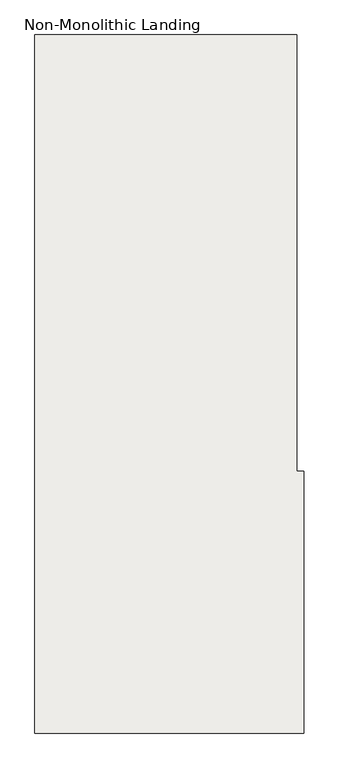
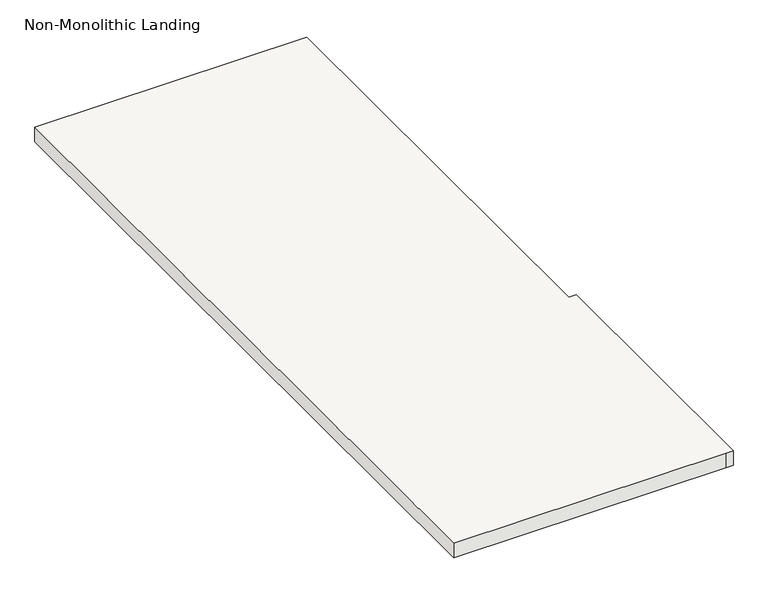
"""IFC4 building model written with IfcOpenShell, lengths in millimetres: slab geometry, Non-Monolithic Landing."""

from ifc_helpers import new_model, si_unit, origin, place, context, project, spatial, faceted_brep, source, transform, mapped, element, save


def non_monolithic_landing_1ab817cb(model_context):
    return source(origin(), model_context, "Body", "Brep", [
        faceted_brep([(-8277.8763529, -1051.6338022, 1809.75), (-8252.4763529, -1051.6338022, 1835.15), (-8252.4763529, -1966.0338022, 1835.15), (-8277.8763529, -1966.0338022, 1809.75), (-9166.8763529, -1051.6338022, 1854.2), (-9166.8763529, -3490.0338022, 1854.2), (-8252.4763529, -3490.0338022, 1854.2), (-8227.0763529, -3490.0338022, 1854.2), (-8227.0763529, -2575.6338022, 1854.2), (-8252.4763529, -2575.6338022, 1854.2), (-8252.4763529, -1051.6338022, 1854.2), (-8277.8763529, -1966.0338022, 1803.4), (-8252.4763529, -1966.0338022, 1803.4), (-8252.4763529, -2575.6338022, 1803.4), (-8227.0763529, -2575.6338022, 1803.4), (-8227.0763529, -3490.0338022, 1803.4), (-8252.4763529, -3490.0338022, 1803.4), (-9166.8763529, -3490.0338022, 1803.4), (-9166.8763529, -1051.6338022, 1803.4), (-8277.8763529, -1051.6338022, 1803.4)], [[[0, 1, 2, 3]], [[4, 5, 6, 7, 8, 9, 10]], [[11, 12, 13, 14, 15, 16, 17, 18, 19]], [[12, 11, 3, 2]], [[11, 19, 0, 3]], [[4, 10, 1, 0, 19, 18]], [[5, 4, 18, 17]], [[6, 5, 17, 16]], [[7, 6, 16, 15]], [[8, 7, 15, 14]], [[9, 8, 14, 13]], [[10, 9, 13, 12, 2, 1]]]),
    ])


if __name__ == "__main__":
    model = new_model("IFC4")
    model_context = context("Model", 3, world=origin())
    ifc_project = project(units=[si_unit("LENGTHUNIT", "METRE", prefix="MILLI")], contexts=[model_context])
    site = spatial("IfcSite", under=ifc_project)
    building = spatial("IfcBuilding", under=site)
    placement = place(None, origin())
    non_monolithic_landing_shape = non_monolithic_landing_1ab817cb(model_context)
    element("IfcSlab", 1, ObjectType="Non-Monolithic Landing", at=placement, inside=building, context=model_context, shape_type="MappedRepresentation", body=[
        mapped(non_monolithic_landing_shape, transform((0.0, 0.0, 0.0), x_axis=(1.0, 0.0, 0.0), y_axis=(0.0, 1.0, 0.0), z_axis=(0.0, 0.0, 1.0))),
    ])
    save(model, "model.ifc")
